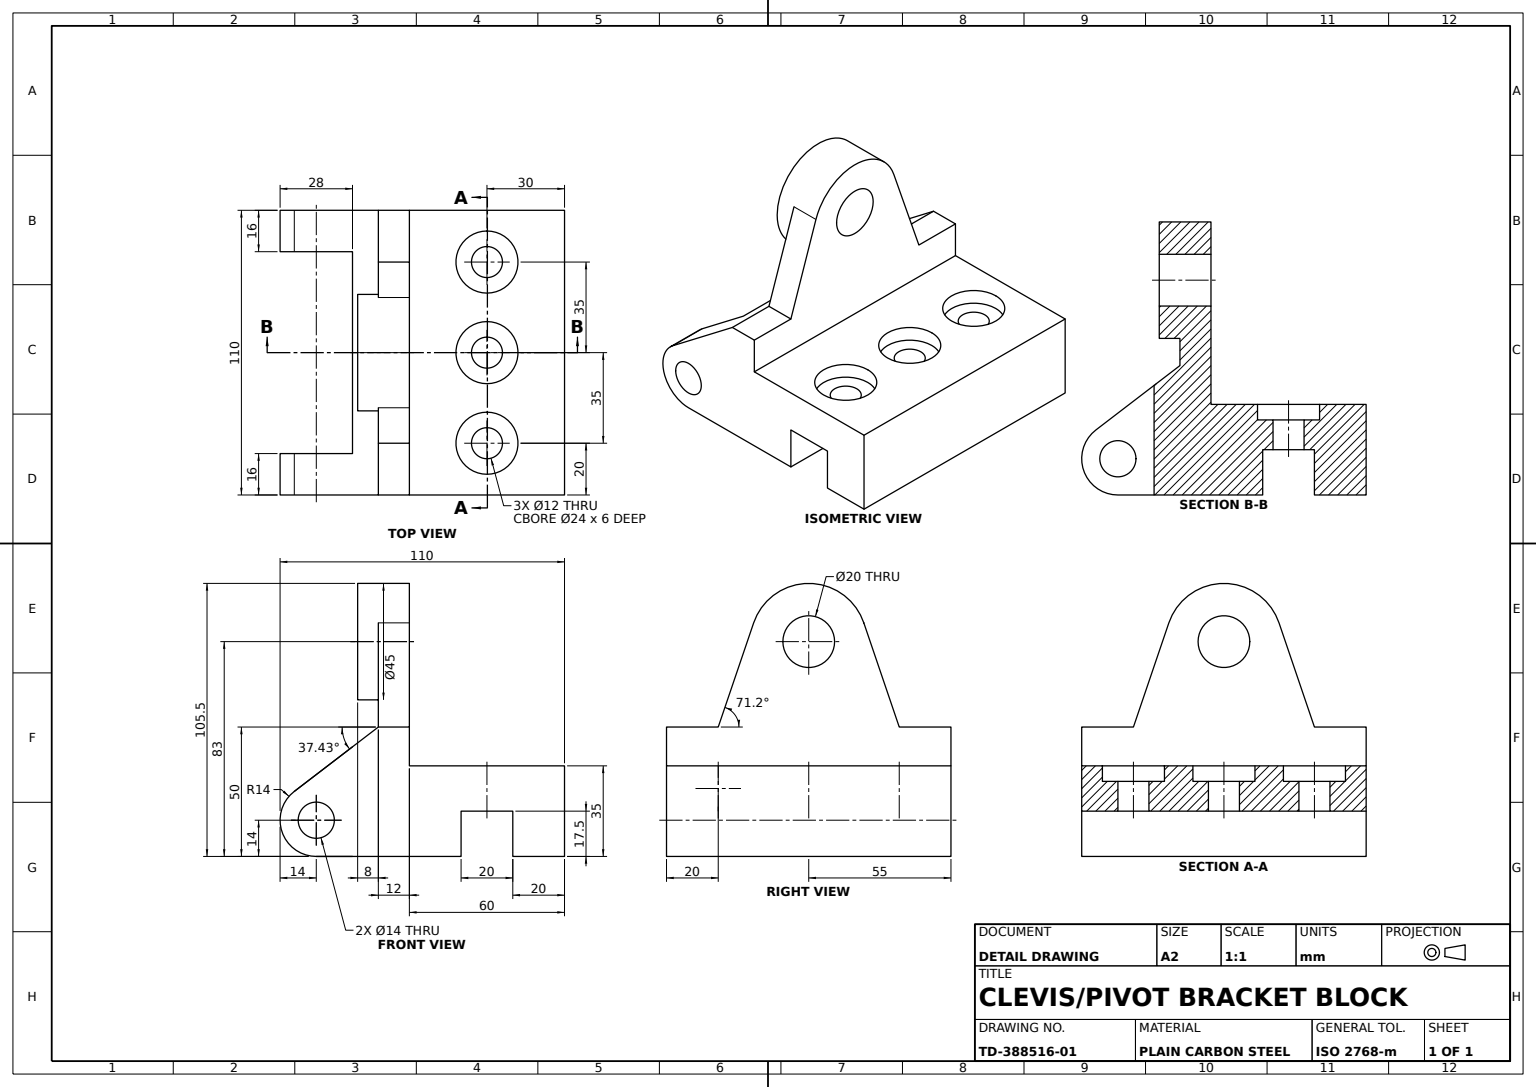
SolidWorks part; units mm, degrees
material "Plain Carbon Steel"
ref_plane "Front Plane" through (0, 0, 0) normal (0, 0, 1) x (1, 0, 0)
ref_plane "Top Plane" through (0, 0, 0) normal (0, 1, 0) x (1, 0, 0)
ref_plane "Right Plane" through (0, 0, 0) normal (1, 0, 0) x (0, 0, -1)
sketch "Base Profile Sketch" plane through (0, 0, 0) normal (0, 0, 1) x (1, 0, 0)
  line L0 (0, -14) -> (56, -14)
  line L1 (56, -14) -> (56, 3.5)
  line L2 (56, 3.5) -> (76, 3.5)
  line L3 (76, 3.5) -> (76, -14)
  line L4 (76, -14) -> (96, -14)
  line L5 (96, -14) -> (96, 21)
  line L6 (96, 21) -> (36, 21)
  line L7 (36, 21) -> (36, 36)
  line L8 (36, 36) -> (24, 36)
  line L9 (24, 36) -> (-8.5092, 11.1173)
  arc A0 (-8.5092, 11.1173) -> (0, -14) centre (0, 0) ccw
  circle A1 centre (0, 0) radius 7
  point P15 (96, 3.5)
  dimension "D1" = 28
  dimension "D7" = 14
  dimension "D2" = 56
  dimension "D3" = 20
  dimension "D4" = 20
  dimension "D5" = 35
  dimension "D6" = 15
  dimension "D8" = 60
  dimension "D9" = 12
extrude "Base Block" add sketch "Base Profile Sketch" against normal mid plane 110
sketch "Guide Slot Sketch" plane through (0, -14, 0) normal (0, -1, 0) x (1, 0, 0)
  line L0 (-14, 55) -> (-14, -55) construction
  line L1 (-14, 39) -> (14, 39)
  line L2 (-14, 39) -> (-14, -39)
  line L3 (-14, -39) -> (14, -39)
  line L4 (14, 39) -> (14, -39)
  line L5 (0, 55) -> (-14, 55) construction
  line L6 (0, -55) -> (56, -55) construction
  line L7 (0, -55) -> (0, 55) construction
  dimension "D1" = 16
  dimension "D2" = 16
  dimension "D3" = 14
extrude "Guide Slot 16x16" cut sketch "Guide Slot Sketch" against normal blind 110
sketch "Pivot Lug Sketch" plane through (36, 0, 0) normal (1, 0, 0) x (0, 0, -1)
  line L0 (0, 0) -> (0, 104.0331) construction
  line L1 (35, 36) -> (21.3, 76.25)
  line L2 (55, 36) -> (-55, 36) construction
  line L3 (-21.3, 76.25) -> (-35, 36)
  line L4 (35, 36) -> (-35, 36)
  line L5 (39, -14) -> (-39, -14) construction
  arc A0 (21.3, 76.25) -> (-21.3, 76.25) centre (0, 69) ccw
  circle A1 centre (0, 69) radius 10
  dimension "D1" = 45
  dimension "D5" = 20
  dimension "D2" = 35
  dimension "D3" = 35
  dimension "D4" = 83
extrude "Pivot Lug" add sketch "Pivot Lug Sketch" against normal blind 12
sketch "Lug Support Sketch" plane through (24, 0, 0) normal (-1, 0, 0) x (0, 0, 1)
  circle A0 centre (0, 69) radius 22.5
  arc A1 (21.3, 76.25) -> (-21.3, 76.25) centre (0, 69) ccw construction
  circle A2 centre (0, 69) radius 10 construction
  circle A3 centre (0, 69) radius 10
  dimension "D1" = 45
extrude "Lug Support Boss" add sketch "Lug Support Sketch" along normal blind 8
hole_wizard "Counterbored Holes 3xØ12" positions "3DSketch1" profile "Sketch6" legacy
sketch3d "3DSketch1"
  line L0 (96, 21, 55) -> (36, 21, 55) construction
  line L1 (96, 21, -55) -> (36, 21, -55) construction
  line L3 (66, 21, 55) -> (66, 21, -55) construction
  line L5 (36, 21, -55) -> (36, 21, 55) construction
  point P0 (66, 21, 35)
  point P2 (66, 21, 0)
  point P4 (66, 21, -35)
  dimension "D1" = 20
  dimension "D2" = 35
  dimension "D3" = 20
  dimension "D4" = 30
sketch "Sketch6" plane through (66, 21, 35) normal (1, 0, 0) x (0, 0, 1)
  line L0 (0, 0) -> (0, 99.8198)
  line L1 (0, 99.8198) -> (6, 99.8198)
  line L2 (6, 99.8198) -> (6, 6)
  line L3 (6, 6) -> (12, 6)
  line L4 (12, 6) -> (12, 0)
  line L5 (12, 0) -> (0, 0)
  line L6 (0, 110) -> (0, -10) construction
  dimension "Diameter" = 12
  dimension "Depth" = 100
  dimension "C-Bore Diameter" = 24
  dimension "C-Bore Depth" = 6
